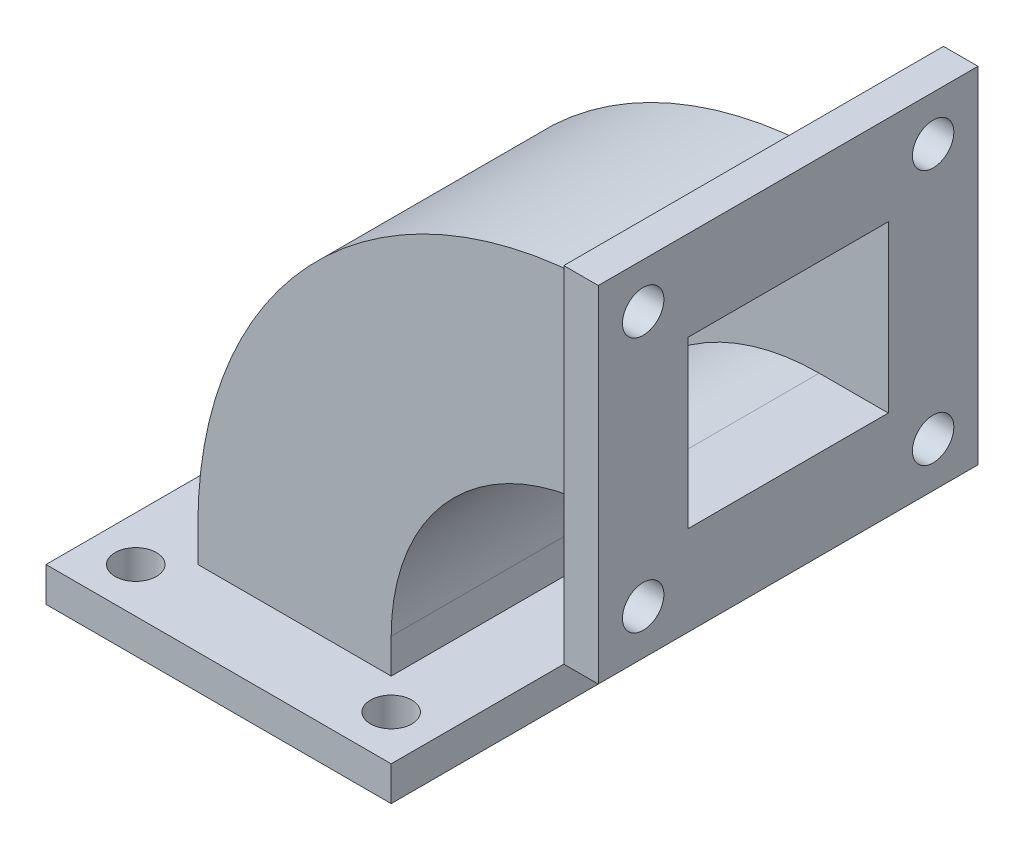
ISO-10303-21;
HEADER;
FILE_DESCRIPTION(('STEP AP214'),'2;1');
FILE_NAME('part.step','',(''),(''),'','','');
FILE_SCHEMA(('AUTOMOTIVE_DESIGN { 1 0 10303 214 1 1 1 1 }'));
ENDSEC;
DATA;
#1=APPLICATION_CONTEXT('core data for automotive mechanical design processes');
#2=APPLICATION_PROTOCOL_DEFINITION('international standard','automotive_design',2000,#1);
#3=PRODUCT_CONTEXT('',#1,'mechanical');
#4=PRODUCT('Part','Part','',(#3));
#5=PRODUCT_RELATED_PRODUCT_CATEGORY('part','',(#4));
#6=PRODUCT_DEFINITION_FORMATION('','',#4);
#7=PRODUCT_DEFINITION_CONTEXT('part definition',#1,'design');
#8=PRODUCT_DEFINITION('design','',#6,#7);
#9=PRODUCT_DEFINITION_SHAPE('','',#8);
#10=(LENGTH_UNIT() NAMED_UNIT(*) SI_UNIT(.MILLI.,.METRE.));
#11=(NAMED_UNIT(*) PLANE_ANGLE_UNIT() SI_UNIT($,.RADIAN.));
#12=(NAMED_UNIT(*) SI_UNIT($,.STERADIAN.) SOLID_ANGLE_UNIT());
#13=UNCERTAINTY_MEASURE_WITH_UNIT(LENGTH_MEASURE(1.E-05),#10,'distance_accuracy_value','');
#14=(GEOMETRIC_REPRESENTATION_CONTEXT(3) GLOBAL_UNCERTAINTY_ASSIGNED_CONTEXT((#13)) GLOBAL_UNIT_ASSIGNED_CONTEXT((#10,
#11,#12)) REPRESENTATION_CONTEXT('',''));
#15=CARTESIAN_POINT('',(0.,0.,0.));
#16=DIRECTION('',(0.,0.,1.));
#17=DIRECTION('',(1.,0.,0.));
#18=AXIS2_PLACEMENT_3D('',#15,#16,#17);
#19=CARTESIAN_POINT('',(5.,0.,0.));
#20=DIRECTION('',(1.,0.,0.));
#21=DIRECTION('',(0.,0.,-1.));
#22=AXIS2_PLACEMENT_3D('',#19,#20,#21);
#23=PLANE('',#22);
#24=CARTESIAN_POINT('',(5.,-18.5,-21.));
#25=DIRECTION('',(1.,0.,0.));
#26=DIRECTION('',(0.,0.,-1.));
#27=AXIS2_PLACEMENT_3D('',#24,#25,#26);
#28=CIRCLE('',#27,2.99999999999999);
#29=CARTESIAN_POINT('',(5.,-18.5,-24.));
#30=VERTEX_POINT('',#29);
#31=EDGE_CURVE('E380',#30,#30,#28,.T.);
#32=ORIENTED_EDGE('',*,*,#31,.F.);
#33=EDGE_LOOP('',(#32));
#34=FACE_BOUND('',#33,.T.);
#35=CARTESIAN_POINT('',(5.,18.5,21.));
#36=DIRECTION('',(1.,0.,0.));
#37=DIRECTION('',(0.,0.,-1.));
#38=AXIS2_PLACEMENT_3D('',#35,#36,#37);
#39=CIRCLE('',#38,3.);
#40=CARTESIAN_POINT('',(5.,18.5,18.));
#41=VERTEX_POINT('',#40);
#42=EDGE_CURVE('E386',#41,#41,#39,.T.);
#43=ORIENTED_EDGE('',*,*,#42,.F.);
#44=EDGE_LOOP('',(#43));
#45=FACE_BOUND('',#44,.T.);
#46=DIRECTION('',(0.,1.,0.));
#47=VECTOR('',#46,1.);
#48=CARTESIAN_POINT('',(5.,25.,-27.5));
#49=LINE('',#48,#47);
#50=CARTESIAN_POINT('',(5.,-25.,-27.5));
#51=VERTEX_POINT('',#50);
#52=CARTESIAN_POINT('',(5.,25.,-27.5));
#53=VERTEX_POINT('',#52);
#54=EDGE_CURVE('E410',#51,#53,#49,.T.);
#55=ORIENTED_EDGE('',*,*,#54,.T.);
#56=DIRECTION('',(0.,0.,1.));
#57=VECTOR('',#56,1.);
#58=CARTESIAN_POINT('',(5.,25.,27.5));
#59=LINE('',#58,#57);
#60=CARTESIAN_POINT('',(5.,25.,27.5));
#61=VERTEX_POINT('',#60);
#62=EDGE_CURVE('E414',#53,#61,#59,.T.);
#63=ORIENTED_EDGE('',*,*,#62,.T.);
#64=DIRECTION('',(0.,-1.,0.));
#65=VECTOR('',#64,1.);
#66=CARTESIAN_POINT('',(5.,25.,27.5));
#67=LINE('',#66,#65);
#68=CARTESIAN_POINT('',(5.,-25.,27.5));
#69=VERTEX_POINT('',#68);
#70=EDGE_CURVE('E418',#61,#69,#67,.T.);
#71=ORIENTED_EDGE('',*,*,#70,.T.);
#72=DIRECTION('',(0.,0.,-1.));
#73=VECTOR('',#72,1.);
#74=CARTESIAN_POINT('',(5.,-25.,27.5));
#75=LINE('',#74,#73);
#76=EDGE_CURVE('E416',#69,#51,#75,.T.);
#77=ORIENTED_EDGE('',*,*,#76,.T.);
#78=EDGE_LOOP('',(#55,#63,#71,#77));
#79=FACE_BOUND('',#78,.T.);
#80=DIRECTION('',(0.,0.,1.));
#81=VECTOR('',#80,1.);
#82=CARTESIAN_POINT('',(5.,12.,14.5));
#83=LINE('',#82,#81);
#84=CARTESIAN_POINT('',(5.,12.,-14.5));
#85=VERTEX_POINT('',#84);
#86=CARTESIAN_POINT('',(5.,12.,14.5));
#87=VERTEX_POINT('',#86);
#88=EDGE_CURVE('E396',#85,#87,#83,.T.);
#89=ORIENTED_EDGE('',*,*,#88,.F.);
#90=DIRECTION('',(0.,1.,0.));
#91=VECTOR('',#90,1.);
#92=CARTESIAN_POINT('',(5.,12.,-14.5));
#93=LINE('',#92,#91);
#94=CARTESIAN_POINT('',(5.,-12.,-14.5));
#95=VERTEX_POINT('',#94);
#96=EDGE_CURVE('E392',#95,#85,#93,.T.);
#97=ORIENTED_EDGE('',*,*,#96,.F.);
#98=DIRECTION('',(0.,0.,-1.));
#99=VECTOR('',#98,1.);
#100=CARTESIAN_POINT('',(5.,-12.,14.5));
#101=LINE('',#100,#99);
#102=CARTESIAN_POINT('',(5.,-12.,14.5));
#103=VERTEX_POINT('',#102);
#104=EDGE_CURVE('E400',#103,#95,#101,.T.);
#105=ORIENTED_EDGE('',*,*,#104,.F.);
#106=DIRECTION('',(0.,-1.,0.));
#107=VECTOR('',#106,1.);
#108=CARTESIAN_POINT('',(5.,12.,14.5));
#109=LINE('',#108,#107);
#110=EDGE_CURVE('E399',#87,#103,#109,.T.);
#111=ORIENTED_EDGE('',*,*,#110,.F.);
#112=EDGE_LOOP('',(#89,#97,#105,#111));
#113=FACE_BOUND('',#112,.T.);
#114=CARTESIAN_POINT('',(5.,18.5,-21.));
#115=DIRECTION('',(1.,0.,0.));
#116=DIRECTION('',(0.,0.,-1.));
#117=AXIS2_PLACEMENT_3D('',#114,#115,#116);
#118=CIRCLE('',#117,3.);
#119=CARTESIAN_POINT('',(5.,18.5,-24.));
#120=VERTEX_POINT('',#119);
#121=EDGE_CURVE('E382',#120,#120,#118,.T.);
#122=ORIENTED_EDGE('',*,*,#121,.F.);
#123=EDGE_LOOP('',(#122));
#124=FACE_BOUND('',#123,.T.);
#125=CARTESIAN_POINT('',(5.,-18.5,21.));
#126=DIRECTION('',(1.,0.,0.));
#127=DIRECTION('',(0.,0.,-1.));
#128=AXIS2_PLACEMENT_3D('',#125,#126,#127);
#129=CIRCLE('',#128,3.);
#130=CARTESIAN_POINT('',(5.,-18.5,18.));
#131=VERTEX_POINT('',#130);
#132=EDGE_CURVE('E371',#131,#131,#129,.T.);
#133=ORIENTED_EDGE('',*,*,#132,.F.);
#134=EDGE_LOOP('',(#133));
#135=FACE_BOUND('',#134,.T.);
#136=ADVANCED_FACE('F44',(#34,#45,#79,#113,#124,#135),#23,.T.);
#137=CARTESIAN_POINT('',(0.,0.,0.));
#138=DIRECTION('',(1.,0.,0.));
#139=DIRECTION('',(0.,0.,-1.));
#140=AXIS2_PLACEMENT_3D('',#137,#138,#139);
#141=PLANE('',#140);
#142=DIRECTION('',(0.,1.,0.));
#143=VECTOR('',#142,1.);
#144=CARTESIAN_POINT('',(0.,-50.,-16.5));
#145=LINE('',#144,#143);
#146=CARTESIAN_POINT('',(0.,-14.,-16.5));
#147=VERTEX_POINT('',#146);
#148=CARTESIAN_POINT('',(0.,14.,-16.5));
#149=VERTEX_POINT('',#148);
#150=EDGE_CURVE('E351',#147,#149,#145,.T.);
#151=ORIENTED_EDGE('',*,*,#150,.T.);
#152=DIRECTION('',(0.,0.,1.));
#153=VECTOR('',#152,1.);
#154=CARTESIAN_POINT('',(0.,14.,0.));
#155=LINE('',#154,#153);
#156=CARTESIAN_POINT('',(0.,14.,16.5));
#157=VERTEX_POINT('',#156);
#158=EDGE_CURVE('E344',#149,#157,#155,.T.);
#159=ORIENTED_EDGE('',*,*,#158,.T.);
#160=DIRECTION('',(0.,-1.,0.));
#161=VECTOR('',#160,1.);
#162=CARTESIAN_POINT('',(0.,-50.,16.5));
#163=LINE('',#162,#161);
#164=CARTESIAN_POINT('',(0.,-14.,16.5));
#165=VERTEX_POINT('',#164);
#166=EDGE_CURVE('E342',#157,#165,#163,.T.);
#167=ORIENTED_EDGE('',*,*,#166,.T.);
#168=DIRECTION('',(0.,0.,-1.));
#169=VECTOR('',#168,1.);
#170=CARTESIAN_POINT('',(0.,-14.,0.));
#171=LINE('',#170,#169);
#172=EDGE_CURVE('E349',#165,#147,#171,.T.);
#173=ORIENTED_EDGE('',*,*,#172,.T.);
#174=EDGE_LOOP('',(#151,#159,#167,#173));
#175=FACE_BOUND('',#174,.T.);
#176=DIRECTION('',(0.,1.,0.));
#177=VECTOR('',#176,1.);
#178=CARTESIAN_POINT('',(0.,25.,-27.5));
#179=LINE('',#178,#177);
#180=CARTESIAN_POINT('',(0.,-25.,-27.5));
#181=VERTEX_POINT('',#180);
#182=CARTESIAN_POINT('',(0.,25.,-27.5));
#183=VERTEX_POINT('',#182);
#184=EDGE_CURVE('E408',#181,#183,#179,.T.);
#185=ORIENTED_EDGE('',*,*,#184,.F.);
#186=DIRECTION('',(0.,0.,-1.));
#187=VECTOR('',#186,1.);
#188=CARTESIAN_POINT('',(0.,-25.,27.5));
#189=LINE('',#188,#187);
#190=CARTESIAN_POINT('',(0.,-25.,27.5));
#191=VERTEX_POINT('',#190);
#192=EDGE_CURVE('E413',#191,#181,#189,.T.);
#193=ORIENTED_EDGE('',*,*,#192,.F.);
#194=DIRECTION('',(0.,-1.,0.));
#195=VECTOR('',#194,1.);
#196=CARTESIAN_POINT('',(0.,25.,27.5));
#197=LINE('',#196,#195);
#198=CARTESIAN_POINT('',(0.,25.,27.5));
#199=VERTEX_POINT('',#198);
#200=EDGE_CURVE('E422',#199,#191,#197,.T.);
#201=ORIENTED_EDGE('',*,*,#200,.F.);
#202=DIRECTION('',(0.,0.,1.));
#203=VECTOR('',#202,1.);
#204=CARTESIAN_POINT('',(0.,25.,27.5));
#205=LINE('',#204,#203);
#206=EDGE_CURVE('E421',#183,#199,#205,.T.);
#207=ORIENTED_EDGE('',*,*,#206,.F.);
#208=EDGE_LOOP('',(#185,#193,#201,#207));
#209=FACE_BOUND('',#208,.T.);
#210=CARTESIAN_POINT('',(0.,18.5,21.));
#211=DIRECTION('',(1.,0.,0.));
#212=DIRECTION('',(0.,0.,-1.));
#213=AXIS2_PLACEMENT_3D('',#210,#211,#212);
#214=CIRCLE('',#213,3.);
#215=CARTESIAN_POINT('',(0.,18.5,18.));
#216=VERTEX_POINT('',#215);
#217=EDGE_CURVE('E387',#216,#216,#214,.T.);
#218=ORIENTED_EDGE('',*,*,#217,.T.);
#219=EDGE_LOOP('',(#218));
#220=FACE_BOUND('',#219,.T.);
#221=CARTESIAN_POINT('',(0.,18.5,-21.));
#222=DIRECTION('',(1.,0.,0.));
#223=DIRECTION('',(0.,0.,-1.));
#224=AXIS2_PLACEMENT_3D('',#221,#222,#223);
#225=CIRCLE('',#224,3.);
#226=CARTESIAN_POINT('',(0.,18.5,-24.));
#227=VERTEX_POINT('',#226);
#228=EDGE_CURVE('E379',#227,#227,#225,.T.);
#229=ORIENTED_EDGE('',*,*,#228,.T.);
#230=EDGE_LOOP('',(#229));
#231=FACE_BOUND('',#230,.T.);
#232=CARTESIAN_POINT('',(0.,-18.5,-21.));
#233=DIRECTION('',(1.,0.,0.));
#234=DIRECTION('',(0.,0.,-1.));
#235=AXIS2_PLACEMENT_3D('',#232,#233,#234);
#236=CIRCLE('',#235,2.99999999999999);
#237=CARTESIAN_POINT('',(0.,-18.5,-24.));
#238=VERTEX_POINT('',#237);
#239=EDGE_CURVE('E372',#238,#238,#236,.T.);
#240=ORIENTED_EDGE('',*,*,#239,.T.);
#241=EDGE_LOOP('',(#240));
#242=FACE_BOUND('',#241,.T.);
#243=CARTESIAN_POINT('',(0.,-18.5,21.));
#244=DIRECTION('',(1.,0.,0.));
#245=DIRECTION('',(0.,0.,-1.));
#246=AXIS2_PLACEMENT_3D('',#243,#244,#245);
#247=CIRCLE('',#246,3.);
#248=CARTESIAN_POINT('',(0.,-18.5,18.));
#249=VERTEX_POINT('',#248);
#250=EDGE_CURVE('E367',#249,#249,#247,.T.);
#251=ORIENTED_EDGE('',*,*,#250,.T.);
#252=EDGE_LOOP('',(#251));
#253=FACE_BOUND('',#252,.T.);
#254=ADVANCED_FACE('F444',(#175,#209,#220,#231,#242,#253),#141,.F.);
#255=CARTESIAN_POINT('',(5.,25.,-27.5));
#256=DIRECTION('',(0.,0.,1.));
#257=DIRECTION('',(0.,-1.,0.));
#258=AXIS2_PLACEMENT_3D('',#255,#256,#257);
#259=PLANE('',#258);
#260=ORIENTED_EDGE('',*,*,#184,.T.);
#261=DIRECTION('',(-1.,0.,0.));
#262=VECTOR('',#261,1.);
#263=CARTESIAN_POINT('',(5.,25.,-27.5));
#264=LINE('',#263,#262);
#265=EDGE_CURVE('E11',#53,#183,#264,.T.);
#266=ORIENTED_EDGE('',*,*,#265,.F.);
#267=ORIENTED_EDGE('',*,*,#54,.F.);
#268=DIRECTION('',(-1.,0.,0.));
#269=VECTOR('',#268,1.);
#270=CARTESIAN_POINT('',(5.,-25.,-27.5));
#271=LINE('',#270,#269);
#272=EDGE_CURVE('E419',#51,#181,#271,.T.);
#273=ORIENTED_EDGE('',*,*,#272,.T.);
#274=EDGE_LOOP('',(#260,#266,#267,#273));
#275=FACE_BOUND('',#274,.T.);
#276=ADVANCED_FACE('F50',(#275),#259,.F.);
#277=CARTESIAN_POINT('',(5.,25.,27.5));
#278=DIRECTION('',(0.,-1.,0.));
#279=DIRECTION('',(0.,0.,-1.));
#280=AXIS2_PLACEMENT_3D('',#277,#278,#279);
#281=PLANE('',#280);
#282=ORIENTED_EDGE('',*,*,#206,.T.);
#283=DIRECTION('',(-1.,0.,0.));
#284=VECTOR('',#283,1.);
#285=CARTESIAN_POINT('',(5.,25.,27.5));
#286=LINE('',#285,#284);
#287=EDGE_CURVE('E52',#61,#199,#286,.T.);
#288=ORIENTED_EDGE('',*,*,#287,.F.);
#289=ORIENTED_EDGE('',*,*,#62,.F.);
#290=ORIENTED_EDGE('',*,*,#265,.T.);
#291=EDGE_LOOP('',(#282,#288,#289,#290));
#292=FACE_BOUND('',#291,.T.);
#293=ADVANCED_FACE('F453',(#292),#281,.F.);
#294=CARTESIAN_POINT('',(5.,25.,27.5));
#295=DIRECTION('',(0.,0.,-1.));
#296=DIRECTION('',(0.,1.,0.));
#297=AXIS2_PLACEMENT_3D('',#294,#295,#296);
#298=PLANE('',#297);
#299=ORIENTED_EDGE('',*,*,#200,.T.);
#300=DIRECTION('',(-1.,0.,0.));
#301=VECTOR('',#300,1.);
#302=CARTESIAN_POINT('',(5.,-25.,27.5));
#303=LINE('',#302,#301);
#304=EDGE_CURVE('E429',#69,#191,#303,.T.);
#305=ORIENTED_EDGE('',*,*,#304,.F.);
#306=ORIENTED_EDGE('',*,*,#70,.F.);
#307=ORIENTED_EDGE('',*,*,#287,.T.);
#308=EDGE_LOOP('',(#299,#305,#306,#307));
#309=FACE_BOUND('',#308,.T.);
#310=ADVANCED_FACE('F440',(#309),#298,.F.);
#311=CARTESIAN_POINT('',(5.,-25.,27.5));
#312=DIRECTION('',(0.,1.,0.));
#313=DIRECTION('',(0.,0.,1.));
#314=AXIS2_PLACEMENT_3D('',#311,#312,#313);
#315=PLANE('',#314);
#316=ORIENTED_EDGE('',*,*,#192,.T.);
#317=ORIENTED_EDGE('',*,*,#272,.F.);
#318=ORIENTED_EDGE('',*,*,#76,.F.);
#319=ORIENTED_EDGE('',*,*,#304,.T.);
#320=EDGE_LOOP('',(#316,#317,#318,#319));
#321=FACE_BOUND('',#320,.T.);
#322=ADVANCED_FACE('F447',(#321),#315,.F.);
#323=CARTESIAN_POINT('',(5.,12.,-14.5));
#324=DIRECTION('',(0.,0.,1.));
#325=DIRECTION('',(0.,-1.,0.));
#326=AXIS2_PLACEMENT_3D('',#323,#324,#325);
#327=PLANE('',#326);
#328=DIRECTION('',(-1.,0.,0.));
#329=VECTOR('',#328,1.);
#330=CARTESIAN_POINT('',(5.,12.,-14.5));
#331=LINE('',#330,#329);
#332=CARTESIAN_POINT('',(-4.99999999999959,12.0000000000004,-14.5));
#333=VERTEX_POINT('',#332);
#334=EDGE_CURVE('E407',#85,#333,#331,.T.);
#335=ORIENTED_EDGE('',*,*,#334,.T.);
#336=CARTESIAN_POINT('',(-4.99999999999999,-45.,-14.5));
#337=DIRECTION('',(0.,0.,-1.));
#338=DIRECTION('',(-1.,0.,0.));
#339=AXIS2_PLACEMENT_3D('',#336,#337,#338);
#340=CIRCLE('',#339,57.0000000000003);
#341=CARTESIAN_POINT('',(-62.,-45.0000000000003,-14.5));
#342=VERTEX_POINT('',#341);
#343=EDGE_CURVE('E217',#342,#333,#340,.T.);
#344=ORIENTED_EDGE('',*,*,#343,.F.);
#345=DIRECTION('',(0.,1.,0.));
#346=VECTOR('',#345,1.);
#347=CARTESIAN_POINT('',(-62.,-50.,-14.5));
#348=LINE('',#347,#346);
#349=CARTESIAN_POINT('',(-62.,-55.,-14.5));
#350=VERTEX_POINT('',#349);
#351=EDGE_CURVE('E221',#350,#342,#348,.T.);
#352=ORIENTED_EDGE('',*,*,#351,.F.);
#353=DIRECTION('',(-1.,0.,0.));
#354=VECTOR('',#353,1.);
#355=CARTESIAN_POINT('',(-62.,-55.,-14.5));
#356=LINE('',#355,#354);
#357=CARTESIAN_POINT('',(-38.,-55.,-14.5));
#358=VERTEX_POINT('',#357);
#359=EDGE_CURVE('E222',#358,#350,#356,.T.);
#360=ORIENTED_EDGE('',*,*,#359,.F.);
#361=DIRECTION('',(0.,1.,0.));
#362=VECTOR('',#361,1.);
#363=CARTESIAN_POINT('',(-38.,-50.,-14.5));
#364=LINE('',#363,#362);
#365=CARTESIAN_POINT('',(-38.,-45.0000000000003,-14.5));
#366=VERTEX_POINT('',#365);
#367=EDGE_CURVE('E210',#358,#366,#364,.T.);
#368=ORIENTED_EDGE('',*,*,#367,.T.);
#369=CARTESIAN_POINT('',(-4.99999999999999,-45.,-14.5));
#370=DIRECTION('',(0.,0.,-1.));
#371=DIRECTION('',(-1.,0.,0.));
#372=AXIS2_PLACEMENT_3D('',#369,#370,#371);
#373=CIRCLE('',#372,33.0000000000003);
#374=CARTESIAN_POINT('',(-4.99999999999975,-11.9999999999997,-14.5));
#375=VERTEX_POINT('',#374);
#376=EDGE_CURVE('E298',#366,#375,#373,.T.);
#377=ORIENTED_EDGE('',*,*,#376,.T.);
#378=DIRECTION('',(-1.,0.,0.));
#379=VECTOR('',#378,1.);
#380=CARTESIAN_POINT('',(5.,-12.,-14.5));
#381=LINE('',#380,#379);
#382=EDGE_CURVE('E405',#95,#375,#381,.T.);
#383=ORIENTED_EDGE('',*,*,#382,.F.);
#384=ORIENTED_EDGE('',*,*,#96,.T.);
#385=EDGE_LOOP('',(#335,#344,#352,#360,#368,#377,#383,#384));
#386=FACE_BOUND('',#385,.T.);
#387=ADVANCED_FACE('F225',(#386),#327,.T.);
#388=CARTESIAN_POINT('',(5.,12.,14.5));
#389=DIRECTION('',(0.,-1.,0.));
#390=DIRECTION('',(0.,0.,-1.));
#391=AXIS2_PLACEMENT_3D('',#388,#389,#390);
#392=PLANE('',#391);
#393=DIRECTION('',(-1.,0.,0.));
#394=VECTOR('',#393,1.);
#395=CARTESIAN_POINT('',(5.,12.,14.5));
#396=LINE('',#395,#394);
#397=CARTESIAN_POINT('',(-4.99999999999959,12.0000000000004,14.5));
#398=VERTEX_POINT('',#397);
#399=EDGE_CURVE('E403',#87,#398,#396,.T.);
#400=ORIENTED_EDGE('',*,*,#399,.T.);
#401=DIRECTION('',(0.,0.,1.));
#402=VECTOR('',#401,1.);
#403=CARTESIAN_POINT('',(-4.99999999999959,12.,-14.5));
#404=LINE('',#403,#402);
#405=EDGE_CURVE('E284',#333,#398,#404,.T.);
#406=ORIENTED_EDGE('',*,*,#405,.F.);
#407=ORIENTED_EDGE('',*,*,#334,.F.);
#408=ORIENTED_EDGE('',*,*,#88,.T.);
#409=EDGE_LOOP('',(#400,#406,#407,#408));
#410=FACE_BOUND('',#409,.T.);
#411=ADVANCED_FACE('F479',(#410),#392,.T.);
#412=CARTESIAN_POINT('',(5.,12.,14.5));
#413=DIRECTION('',(0.,0.,-1.));
#414=DIRECTION('',(0.,1.,0.));
#415=AXIS2_PLACEMENT_3D('',#412,#413,#414);
#416=PLANE('',#415);
#417=DIRECTION('',(-1.,0.,0.));
#418=VECTOR('',#417,1.);
#419=CARTESIAN_POINT('',(5.,-12.,14.5));
#420=LINE('',#419,#418);
#421=CARTESIAN_POINT('',(-4.99999999999975,-11.9999999999997,14.5));
#422=VERTEX_POINT('',#421);
#423=EDGE_CURVE('E69',#103,#422,#420,.T.);
#424=ORIENTED_EDGE('',*,*,#423,.T.);
#425=CARTESIAN_POINT('',(-4.99999999999999,-45.,14.5));
#426=DIRECTION('',(0.,0.,-1.));
#427=DIRECTION('',(-1.,0.,0.));
#428=AXIS2_PLACEMENT_3D('',#425,#426,#427);
#429=CIRCLE('',#428,33.0000000000003);
#430=CARTESIAN_POINT('',(-38.,-45.0000000000003,14.5));
#431=VERTEX_POINT('',#430);
#432=EDGE_CURVE('E288',#431,#422,#429,.T.);
#433=ORIENTED_EDGE('',*,*,#432,.F.);
#434=DIRECTION('',(0.,1.,0.));
#435=VECTOR('',#434,1.);
#436=CARTESIAN_POINT('',(-38.,-50.,14.5));
#437=LINE('',#436,#435);
#438=CARTESIAN_POINT('',(-38.,-55.,14.5));
#439=VERTEX_POINT('',#438);
#440=EDGE_CURVE('E281',#439,#431,#437,.T.);
#441=ORIENTED_EDGE('',*,*,#440,.F.);
#442=DIRECTION('',(1.,0.,0.));
#443=VECTOR('',#442,1.);
#444=CARTESIAN_POINT('',(-62.,-55.,14.5));
#445=LINE('',#444,#443);
#446=CARTESIAN_POINT('',(-62.,-55.,14.5));
#447=VERTEX_POINT('',#446);
#448=EDGE_CURVE('E234',#447,#439,#445,.T.);
#449=ORIENTED_EDGE('',*,*,#448,.F.);
#450=DIRECTION('',(0.,1.,0.));
#451=VECTOR('',#450,1.);
#452=CARTESIAN_POINT('',(-62.,-50.,14.5));
#453=LINE('',#452,#451);
#454=CARTESIAN_POINT('',(-62.,-45.0000000000003,14.5));
#455=VERTEX_POINT('',#454);
#456=EDGE_CURVE('E279',#447,#455,#453,.T.);
#457=ORIENTED_EDGE('',*,*,#456,.T.);
#458=CARTESIAN_POINT('',(-4.99999999999999,-45.,14.5));
#459=DIRECTION('',(0.,0.,-1.));
#460=DIRECTION('',(-1.,0.,0.));
#461=AXIS2_PLACEMENT_3D('',#458,#459,#460);
#462=CIRCLE('',#461,57.0000000000003);
#463=EDGE_CURVE('E286',#455,#398,#462,.T.);
#464=ORIENTED_EDGE('',*,*,#463,.T.);
#465=ORIENTED_EDGE('',*,*,#399,.F.);
#466=ORIENTED_EDGE('',*,*,#110,.T.);
#467=EDGE_LOOP('',(#424,#433,#441,#449,#457,#464,#465,#466));
#468=FACE_BOUND('',#467,.T.);
#469=ADVANCED_FACE('F482',(#468),#416,.T.);
#470=CARTESIAN_POINT('',(5.,-12.,14.5));
#471=DIRECTION('',(0.,1.,0.));
#472=DIRECTION('',(0.,0.,1.));
#473=AXIS2_PLACEMENT_3D('',#470,#471,#472);
#474=PLANE('',#473);
#475=ORIENTED_EDGE('',*,*,#382,.T.);
#476=DIRECTION('',(0.,0.,-1.));
#477=VECTOR('',#476,1.);
#478=CARTESIAN_POINT('',(-4.99999999999975,-12.,-14.5));
#479=LINE('',#478,#477);
#480=EDGE_CURVE('E293',#422,#375,#479,.T.);
#481=ORIENTED_EDGE('',*,*,#480,.F.);
#482=ORIENTED_EDGE('',*,*,#423,.F.);
#483=ORIENTED_EDGE('',*,*,#104,.T.);
#484=EDGE_LOOP('',(#475,#481,#482,#483));
#485=FACE_BOUND('',#484,.T.);
#486=ADVANCED_FACE('F489',(#485),#474,.T.);
#487=CARTESIAN_POINT('',(5.,18.5,21.));
#488=DIRECTION('',(-1.,0.,0.));
#489=DIRECTION('',(0.,0.,1.));
#490=AXIS2_PLACEMENT_3D('',#487,#488,#489);
#491=CYLINDRICAL_SURFACE('',#490,3.);
#492=ORIENTED_EDGE('',*,*,#42,.T.);
#493=EDGE_LOOP('',(#492));
#494=FACE_BOUND('',#493,.T.);
#495=ORIENTED_EDGE('',*,*,#217,.F.);
#496=EDGE_LOOP('',(#495));
#497=FACE_BOUND('',#496,.T.);
#498=ADVANCED_FACE('F497',(#494,#497),#491,.F.);
#499=CARTESIAN_POINT('',(5.,18.5,-21.));
#500=DIRECTION('',(-1.,0.,0.));
#501=DIRECTION('',(0.,0.,1.));
#502=AXIS2_PLACEMENT_3D('',#499,#500,#501);
#503=CYLINDRICAL_SURFACE('',#502,3.);
#504=ORIENTED_EDGE('',*,*,#121,.T.);
#505=EDGE_LOOP('',(#504));
#506=FACE_BOUND('',#505,.T.);
#507=ORIENTED_EDGE('',*,*,#228,.F.);
#508=EDGE_LOOP('',(#507));
#509=FACE_BOUND('',#508,.T.);
#510=ADVANCED_FACE('F496',(#506,#509),#503,.F.);
#511=CARTESIAN_POINT('',(5.,-18.5,-21.));
#512=DIRECTION('',(-1.,0.,0.));
#513=DIRECTION('',(0.,0.,1.));
#514=AXIS2_PLACEMENT_3D('',#511,#512,#513);
#515=CYLINDRICAL_SURFACE('',#514,2.99999999999999);
#516=ORIENTED_EDGE('',*,*,#31,.T.);
#517=EDGE_LOOP('',(#516));
#518=FACE_BOUND('',#517,.T.);
#519=ORIENTED_EDGE('',*,*,#239,.F.);
#520=EDGE_LOOP('',(#519));
#521=FACE_BOUND('',#520,.T.);
#522=ADVANCED_FACE('F504',(#518,#521),#515,.F.);
#523=CARTESIAN_POINT('',(5.,-18.5,21.));
#524=DIRECTION('',(-1.,0.,0.));
#525=DIRECTION('',(0.,0.,1.));
#526=AXIS2_PLACEMENT_3D('',#523,#524,#525);
#527=CYLINDRICAL_SURFACE('',#526,3.);
#528=ORIENTED_EDGE('',*,*,#132,.T.);
#529=EDGE_LOOP('',(#528));
#530=FACE_BOUND('',#529,.T.);
#531=ORIENTED_EDGE('',*,*,#250,.F.);
#532=EDGE_LOOP('',(#531));
#533=FACE_BOUND('',#532,.T.);
#534=ADVANCED_FACE('F507',(#530,#533),#527,.F.);
#535=CARTESIAN_POINT('',(-64.,-50.,-14.5));
#536=DIRECTION('',(-1.,0.,0.));
#537=DIRECTION('',(0.,0.,1.));
#538=AXIS2_PLACEMENT_3D('',#535,#536,#537);
#539=PLANE('',#538);
#540=DIRECTION('',(0.,1.,0.));
#541=VECTOR('',#540,1.);
#542=CARTESIAN_POINT('',(-64.,-50.,16.5));
#543=LINE('',#542,#541);
#544=CARTESIAN_POINT('',(-64.,-50.,16.5));
#545=VERTEX_POINT('',#544);
#546=CARTESIAN_POINT('',(-64.0000000000002,-45.0000000000001,16.5));
#547=VERTEX_POINT('',#546);
#548=EDGE_CURVE('E302',#545,#547,#543,.T.);
#549=ORIENTED_EDGE('',*,*,#548,.T.);
#550=DIRECTION('',(0.,0.,-1.));
#551=VECTOR('',#550,1.);
#552=CARTESIAN_POINT('',(-64.0000000000003,-45.0000000000003,0.));
#553=LINE('',#552,#551);
#554=CARTESIAN_POINT('',(-64.0000000000002,-45.0000000000001,-16.5));
#555=VERTEX_POINT('',#554);
#556=EDGE_CURVE('E308',#555,#547,#553,.F.);
#557=ORIENTED_EDGE('',*,*,#556,.F.);
#558=DIRECTION('',(0.,1.,0.));
#559=VECTOR('',#558,1.);
#560=CARTESIAN_POINT('',(-64.,-50.,-16.5));
#561=LINE('',#560,#559);
#562=CARTESIAN_POINT('',(-64.,-50.,-16.5));
#563=VERTEX_POINT('',#562);
#564=EDGE_CURVE('E310',#563,#555,#561,.T.);
#565=ORIENTED_EDGE('',*,*,#564,.F.);
#566=DIRECTION('',(0.,0.,1.));
#567=VECTOR('',#566,1.);
#568=CARTESIAN_POINT('',(-64.,-50.,0.));
#569=LINE('',#568,#567);
#570=EDGE_CURVE('E301',#563,#545,#569,.T.);
#571=ORIENTED_EDGE('',*,*,#570,.T.);
#572=EDGE_LOOP('',(#549,#557,#565,#571));
#573=FACE_BOUND('',#572,.T.);
#574=ADVANCED_FACE('F512',(#573),#539,.T.);
#575=CARTESIAN_POINT('',(-62.,-50.,16.5));
#576=DIRECTION('',(0.,0.,1.));
#577=DIRECTION('',(1.,0.,0.));
#578=AXIS2_PLACEMENT_3D('',#575,#576,#577);
#579=PLANE('',#578);
#580=DIRECTION('',(0.,1.,0.));
#581=VECTOR('',#580,1.);
#582=CARTESIAN_POINT('',(-36.,-50.,16.5));
#583=LINE('',#582,#581);
#584=CARTESIAN_POINT('',(-36.,-50.,16.5));
#585=VERTEX_POINT('',#584);
#586=CARTESIAN_POINT('',(-36.0000000000002,-45.0000000000001,16.5));
#587=VERTEX_POINT('',#586);
#588=EDGE_CURVE('E305',#585,#587,#583,.T.);
#589=ORIENTED_EDGE('',*,*,#588,.T.);
#590=CARTESIAN_POINT('',(-4.99999999999999,-45.,16.5));
#591=DIRECTION('',(0.,0.,1.));
#592=DIRECTION('',(1.,0.,0.));
#593=AXIS2_PLACEMENT_3D('',#590,#591,#592);
#594=CIRCLE('',#593,31.0000000000003);
#595=CARTESIAN_POINT('',(-4.99999999999979,-14.,16.5));
#596=VERTEX_POINT('',#595);
#597=EDGE_CURVE('E324',#587,#596,#594,.F.);
#598=ORIENTED_EDGE('',*,*,#597,.T.);
#599=DIRECTION('',(1.,0.,0.));
#600=VECTOR('',#599,1.);
#601=CARTESIAN_POINT('',(-4.99999999999967,-14.,16.5));
#602=LINE('',#601,#600);
#603=EDGE_CURVE('E347',#596,#165,#602,.T.);
#604=ORIENTED_EDGE('',*,*,#603,.T.);
#605=ORIENTED_EDGE('',*,*,#166,.F.);
#606=DIRECTION('',(1.,0.,0.));
#607=VECTOR('',#606,1.);
#608=CARTESIAN_POINT('',(-4.99999999999967,14.,16.5));
#609=LINE('',#608,#607);
#610=CARTESIAN_POINT('',(-4.99999999999979,14.0000000000002,16.5));
#611=VERTEX_POINT('',#610);
#612=EDGE_CURVE('E338',#611,#157,#609,.T.);
#613=ORIENTED_EDGE('',*,*,#612,.F.);
#614=CARTESIAN_POINT('',(-4.99999999999999,-45.,16.5));
#615=DIRECTION('',(0.,0.,1.));
#616=DIRECTION('',(1.,0.,0.));
#617=AXIS2_PLACEMENT_3D('',#614,#615,#616);
#618=CIRCLE('',#617,59.0000000000003);
#619=EDGE_CURVE('E325',#547,#611,#618,.F.);
#620=ORIENTED_EDGE('',*,*,#619,.F.);
#621=ORIENTED_EDGE('',*,*,#548,.F.);
#622=DIRECTION('',(1.,0.,0.));
#623=VECTOR('',#622,1.);
#624=CARTESIAN_POINT('',(0.,-50.,16.5));
#625=LINE('',#624,#623);
#626=EDGE_CURVE('E353',#545,#585,#625,.T.);
#627=ORIENTED_EDGE('',*,*,#626,.T.);
#628=EDGE_LOOP('',(#589,#598,#604,#605,#613,#620,#621,#627));
#629=FACE_BOUND('',#628,.T.);
#630=ADVANCED_FACE('F536',(#629),#579,.T.);
#631=CARTESIAN_POINT('',(-36.,-50.,-14.5));
#632=DIRECTION('',(1.,0.,0.));
#633=DIRECTION('',(0.,0.,-1.));
#634=AXIS2_PLACEMENT_3D('',#631,#632,#633);
#635=PLANE('',#634);
#636=DIRECTION('',(0.,1.,0.));
#637=VECTOR('',#636,1.);
#638=CARTESIAN_POINT('',(-36.,-50.,-16.5));
#639=LINE('',#638,#637);
#640=CARTESIAN_POINT('',(-36.,-50.,-16.5));
#641=VERTEX_POINT('',#640);
#642=CARTESIAN_POINT('',(-36.0000000000002,-45.0000000000001,-16.5));
#643=VERTEX_POINT('',#642);
#644=EDGE_CURVE('E316',#641,#643,#639,.T.);
#645=ORIENTED_EDGE('',*,*,#644,.T.);
#646=DIRECTION('',(0.,0.,-1.));
#647=VECTOR('',#646,1.);
#648=CARTESIAN_POINT('',(-36.0000000000003,-45.0000000000003,0.));
#649=LINE('',#648,#647);
#650=EDGE_CURVE('E312',#587,#643,#649,.T.);
#651=ORIENTED_EDGE('',*,*,#650,.F.);
#652=ORIENTED_EDGE('',*,*,#588,.F.);
#653=DIRECTION('',(0.,0.,-1.));
#654=VECTOR('',#653,1.);
#655=CARTESIAN_POINT('',(-36.,-50.,0.));
#656=LINE('',#655,#654);
#657=EDGE_CURVE('E357',#585,#641,#656,.T.);
#658=ORIENTED_EDGE('',*,*,#657,.T.);
#659=EDGE_LOOP('',(#645,#651,#652,#658));
#660=FACE_BOUND('',#659,.T.);
#661=ADVANCED_FACE('F535',(#660),#635,.T.);
#662=CARTESIAN_POINT('',(-62.,-50.,-16.5));
#663=DIRECTION('',(0.,0.,-1.));
#664=DIRECTION('',(-1.,0.,0.));
#665=AXIS2_PLACEMENT_3D('',#662,#663,#664);
#666=PLANE('',#665);
#667=ORIENTED_EDGE('',*,*,#564,.T.);
#668=CARTESIAN_POINT('',(-4.99999999999999,-45.,-16.5));
#669=DIRECTION('',(0.,0.,-1.));
#670=DIRECTION('',(-1.,0.,0.));
#671=AXIS2_PLACEMENT_3D('',#668,#669,#670);
#672=CIRCLE('',#671,59.0000000000003);
#673=CARTESIAN_POINT('',(-4.99999999999979,14.,-16.5));
#674=VERTEX_POINT('',#673);
#675=EDGE_CURVE('E317',#555,#674,#672,.T.);
#676=ORIENTED_EDGE('',*,*,#675,.T.);
#677=DIRECTION('',(1.,0.,0.));
#678=VECTOR('',#677,1.);
#679=CARTESIAN_POINT('',(-4.99999999999967,14.,-16.5));
#680=LINE('',#679,#678);
#681=EDGE_CURVE('E337',#674,#149,#680,.T.);
#682=ORIENTED_EDGE('',*,*,#681,.T.);
#683=ORIENTED_EDGE('',*,*,#150,.F.);
#684=DIRECTION('',(1.,0.,0.));
#685=VECTOR('',#684,1.);
#686=CARTESIAN_POINT('',(-4.99999999999967,-14.,-16.5));
#687=LINE('',#686,#685);
#688=CARTESIAN_POINT('',(-4.99999999999987,-13.9999999999998,-16.5));
#689=VERTEX_POINT('',#688);
#690=EDGE_CURVE('E58',#689,#147,#687,.T.);
#691=ORIENTED_EDGE('',*,*,#690,.F.);
#692=CARTESIAN_POINT('',(-4.99999999999999,-45.,-16.5));
#693=DIRECTION('',(0.,0.,-1.));
#694=DIRECTION('',(-1.,0.,0.));
#695=AXIS2_PLACEMENT_3D('',#692,#693,#694);
#696=CIRCLE('',#695,31.0000000000003);
#697=EDGE_CURVE('E331',#643,#689,#696,.T.);
#698=ORIENTED_EDGE('',*,*,#697,.F.);
#699=ORIENTED_EDGE('',*,*,#644,.F.);
#700=DIRECTION('',(-1.,0.,0.));
#701=VECTOR('',#700,1.);
#702=CARTESIAN_POINT('',(0.,-50.,-16.5));
#703=LINE('',#702,#701);
#704=EDGE_CURVE('E315',#641,#563,#703,.T.);
#705=ORIENTED_EDGE('',*,*,#704,.T.);
#706=EDGE_LOOP('',(#667,#676,#682,#683,#691,#698,#699,#705));
#707=FACE_BOUND('',#706,.T.);
#708=ADVANCED_FACE('F526',(#707),#666,.T.);
#709=CARTESIAN_POINT('',(-4.99999999999999,-45.,0.));
#710=DIRECTION('',(0.,0.,-1.));
#711=DIRECTION('',(-1.,0.,0.));
#712=AXIS2_PLACEMENT_3D('',#709,#710,#711);
#713=CYLINDRICAL_SURFACE('',#712,59.0000000000003);
#714=ORIENTED_EDGE('',*,*,#619,.T.);
#715=DIRECTION('',(0.,0.,1.));
#716=VECTOR('',#715,1.);
#717=CARTESIAN_POINT('',(-4.99999999999959,14.,-14.5));
#718=LINE('',#717,#716);
#719=EDGE_CURVE('E326',#674,#611,#718,.T.);
#720=ORIENTED_EDGE('',*,*,#719,.F.);
#721=ORIENTED_EDGE('',*,*,#675,.F.);
#722=ORIENTED_EDGE('',*,*,#556,.T.);
#723=EDGE_LOOP('',(#714,#720,#721,#722));
#724=FACE_BOUND('',#723,.T.);
#725=ADVANCED_FACE('F523',(#724),#713,.T.);
#726=CARTESIAN_POINT('',(-4.99999999999999,-45.,0.));
#727=DIRECTION('',(0.,0.,-1.));
#728=DIRECTION('',(-1.,0.,0.));
#729=AXIS2_PLACEMENT_3D('',#726,#727,#728);
#730=CYLINDRICAL_SURFACE('',#729,31.0000000000003);
#731=ORIENTED_EDGE('',*,*,#697,.T.);
#732=DIRECTION('',(0.,0.,-1.));
#733=VECTOR('',#732,1.);
#734=CARTESIAN_POINT('',(-4.99999999999975,-14.,-14.5));
#735=LINE('',#734,#733);
#736=EDGE_CURVE('E334',#596,#689,#735,.T.);
#737=ORIENTED_EDGE('',*,*,#736,.F.);
#738=ORIENTED_EDGE('',*,*,#597,.F.);
#739=ORIENTED_EDGE('',*,*,#650,.T.);
#740=EDGE_LOOP('',(#731,#737,#738,#739));
#741=FACE_BOUND('',#740,.T.);
#742=ADVANCED_FACE('F520',(#741),#730,.F.);
#743=CARTESIAN_POINT('',(-4.99999999999967,14.,-14.5));
#744=DIRECTION('',(0.,1.,0.));
#745=DIRECTION('',(0.,0.,1.));
#746=AXIS2_PLACEMENT_3D('',#743,#744,#745);
#747=PLANE('',#746);
#748=ORIENTED_EDGE('',*,*,#612,.T.);
#749=ORIENTED_EDGE('',*,*,#158,.F.);
#750=ORIENTED_EDGE('',*,*,#681,.F.);
#751=ORIENTED_EDGE('',*,*,#719,.T.);
#752=EDGE_LOOP('',(#748,#749,#750,#751));
#753=FACE_BOUND('',#752,.T.);
#754=ADVANCED_FACE('F517',(#753),#747,.T.);
#755=CARTESIAN_POINT('',(-4.99999999999967,-14.,-14.5));
#756=DIRECTION('',(0.,-1.,0.));
#757=DIRECTION('',(0.,0.,-1.));
#758=AXIS2_PLACEMENT_3D('',#755,#756,#757);
#759=PLANE('',#758);
#760=ORIENTED_EDGE('',*,*,#690,.T.);
#761=ORIENTED_EDGE('',*,*,#172,.F.);
#762=ORIENTED_EDGE('',*,*,#603,.F.);
#763=ORIENTED_EDGE('',*,*,#736,.T.);
#764=EDGE_LOOP('',(#760,#761,#762,#763));
#765=FACE_BOUND('',#764,.T.);
#766=ADVANCED_FACE('F511',(#765),#759,.T.);
#767=CARTESIAN_POINT('',(-62.,-50.,-14.5));
#768=DIRECTION('',(-1.,0.,0.));
#769=DIRECTION('',(0.,0.,1.));
#770=AXIS2_PLACEMENT_3D('',#767,#768,#769);
#771=PLANE('',#770);
#772=ORIENTED_EDGE('',*,*,#456,.F.);
#773=DIRECTION('',(0.,0.,1.));
#774=VECTOR('',#773,1.);
#775=CARTESIAN_POINT('',(-62.,-55.,-14.5));
#776=LINE('',#775,#774);
#777=EDGE_CURVE('E229',#350,#447,#776,.T.);
#778=ORIENTED_EDGE('',*,*,#777,.F.);
#779=ORIENTED_EDGE('',*,*,#351,.T.);
#780=DIRECTION('',(0.,0.,1.));
#781=VECTOR('',#780,1.);
#782=CARTESIAN_POINT('',(-62.,-45.0000000000003,-14.5));
#783=LINE('',#782,#781);
#784=EDGE_CURVE('E274',#342,#455,#783,.T.);
#785=ORIENTED_EDGE('',*,*,#784,.T.);
#786=EDGE_LOOP('',(#772,#778,#779,#785));
#787=FACE_BOUND('',#786,.T.);
#788=ADVANCED_FACE('F516',(#787),#771,.F.);
#789=CARTESIAN_POINT('',(-38.,-50.,-14.5));
#790=DIRECTION('',(1.,0.,0.));
#791=DIRECTION('',(0.,0.,-1.));
#792=AXIS2_PLACEMENT_3D('',#789,#790,#791);
#793=PLANE('',#792);
#794=ORIENTED_EDGE('',*,*,#367,.F.);
#795=DIRECTION('',(0.,0.,-1.));
#796=VECTOR('',#795,1.);
#797=CARTESIAN_POINT('',(-38.,-55.,-14.5));
#798=LINE('',#797,#796);
#799=EDGE_CURVE('E215',#439,#358,#798,.T.);
#800=ORIENTED_EDGE('',*,*,#799,.F.);
#801=ORIENTED_EDGE('',*,*,#440,.T.);
#802=DIRECTION('',(0.,0.,-1.));
#803=VECTOR('',#802,1.);
#804=CARTESIAN_POINT('',(-38.,-45.0000000000003,-14.5));
#805=LINE('',#804,#803);
#806=EDGE_CURVE('E214',#431,#366,#805,.T.);
#807=ORIENTED_EDGE('',*,*,#806,.T.);
#808=EDGE_LOOP('',(#794,#800,#801,#807));
#809=FACE_BOUND('',#808,.T.);
#810=ADVANCED_FACE('F207',(#809),#793,.F.);
#811=CARTESIAN_POINT('',(-4.99999999999999,-45.,0.));
#812=DIRECTION('',(0.,0.,-1.));
#813=DIRECTION('',(-1.,0.,0.));
#814=AXIS2_PLACEMENT_3D('',#811,#812,#813);
#815=CYLINDRICAL_SURFACE('',#814,57.0000000000003);
#816=ORIENTED_EDGE('',*,*,#463,.F.);
#817=ORIENTED_EDGE('',*,*,#784,.F.);
#818=ORIENTED_EDGE('',*,*,#343,.T.);
#819=ORIENTED_EDGE('',*,*,#405,.T.);
#820=EDGE_LOOP('',(#816,#817,#818,#819));
#821=FACE_BOUND('',#820,.T.);
#822=ADVANCED_FACE('F547',(#821),#815,.F.);
#823=CARTESIAN_POINT('',(-4.99999999999999,-45.,0.));
#824=DIRECTION('',(0.,0.,-1.));
#825=DIRECTION('',(-1.,0.,0.));
#826=AXIS2_PLACEMENT_3D('',#823,#824,#825);
#827=CYLINDRICAL_SURFACE('',#826,33.0000000000003);
#828=ORIENTED_EDGE('',*,*,#376,.F.);
#829=ORIENTED_EDGE('',*,*,#806,.F.);
#830=ORIENTED_EDGE('',*,*,#432,.T.);
#831=ORIENTED_EDGE('',*,*,#480,.T.);
#832=EDGE_LOOP('',(#828,#829,#830,#831));
#833=FACE_BOUND('',#832,.T.);
#834=ADVANCED_FACE('F542',(#833),#827,.T.);
#835=CARTESIAN_POINT('',(0.,-50.,0.));
#836=DIRECTION('',(0.,1.,0.));
#837=DIRECTION('',(0.,0.,1.));
#838=AXIS2_PLACEMENT_3D('',#835,#836,#837);
#839=PLANE('',#838);
#840=DIRECTION('',(0.,0.,-1.));
#841=VECTOR('',#840,1.);
#842=CARTESIAN_POINT('',(-25.,-50.,-27.5));
#843=LINE('',#842,#841);
#844=CARTESIAN_POINT('',(-25.,-50.,27.5));
#845=VERTEX_POINT('',#844);
#846=CARTESIAN_POINT('',(-25.,-50.,-27.5));
#847=VERTEX_POINT('',#846);
#848=EDGE_CURVE('E244',#845,#847,#843,.T.);
#849=ORIENTED_EDGE('',*,*,#848,.T.);
#850=DIRECTION('',(-1.,0.,0.));
#851=VECTOR('',#850,1.);
#852=CARTESIAN_POINT('',(-75.,-50.,-27.5));
#853=LINE('',#852,#851);
#854=CARTESIAN_POINT('',(-75.,-50.,-27.5));
#855=VERTEX_POINT('',#854);
#856=EDGE_CURVE('E257',#847,#855,#853,.T.);
#857=ORIENTED_EDGE('',*,*,#856,.T.);
#858=DIRECTION('',(0.,0.,1.));
#859=VECTOR('',#858,1.);
#860=CARTESIAN_POINT('',(-75.,-50.,-27.5));
#861=LINE('',#860,#859);
#862=CARTESIAN_POINT('',(-75.,-50.,27.5));
#863=VERTEX_POINT('',#862);
#864=EDGE_CURVE('E263',#855,#863,#861,.T.);
#865=ORIENTED_EDGE('',*,*,#864,.T.);
#866=DIRECTION('',(1.,0.,0.));
#867=VECTOR('',#866,1.);
#868=CARTESIAN_POINT('',(-75.,-50.,27.5));
#869=LINE('',#868,#867);
#870=EDGE_CURVE('E249',#863,#845,#869,.T.);
#871=ORIENTED_EDGE('',*,*,#870,.T.);
#872=EDGE_LOOP('',(#849,#857,#865,#871));
#873=FACE_BOUND('',#872,.T.);
#874=CARTESIAN_POINT('',(-68.5,-50.,-21.));
#875=DIRECTION('',(0.,1.,0.));
#876=DIRECTION('',(0.,0.,1.));
#877=AXIS2_PLACEMENT_3D('',#874,#875,#876);
#878=CIRCLE('',#877,3.00000000000001);
#879=CARTESIAN_POINT('',(-68.5,-50.,-18.));
#880=VERTEX_POINT('',#879);
#881=EDGE_CURVE('E240',#880,#880,#878,.T.);
#882=ORIENTED_EDGE('',*,*,#881,.F.);
#883=EDGE_LOOP('',(#882));
#884=FACE_BOUND('',#883,.T.);
#885=CARTESIAN_POINT('',(-31.5,-50.,-21.));
#886=DIRECTION('',(0.,1.,0.));
#887=DIRECTION('',(0.,0.,1.));
#888=AXIS2_PLACEMENT_3D('',#885,#886,#887);
#889=CIRCLE('',#888,3.);
#890=CARTESIAN_POINT('',(-31.5,-50.,-18.));
#891=VERTEX_POINT('',#890);
#892=EDGE_CURVE('E612',#891,#891,#889,.T.);
#893=ORIENTED_EDGE('',*,*,#892,.F.);
#894=EDGE_LOOP('',(#893));
#895=FACE_BOUND('',#894,.T.);
#896=CARTESIAN_POINT('',(-31.5,-50.,21.));
#897=DIRECTION('',(0.,1.,0.));
#898=DIRECTION('',(0.,0.,1.));
#899=AXIS2_PLACEMENT_3D('',#896,#897,#898);
#900=CIRCLE('',#899,3.);
#901=CARTESIAN_POINT('',(-31.5,-50.,24.));
#902=VERTEX_POINT('',#901);
#903=EDGE_CURVE('E607',#902,#902,#900,.T.);
#904=ORIENTED_EDGE('',*,*,#903,.F.);
#905=EDGE_LOOP('',(#904));
#906=FACE_BOUND('',#905,.T.);
#907=CARTESIAN_POINT('',(-68.5,-50.,21.));
#908=DIRECTION('',(0.,1.,0.));
#909=DIRECTION('',(0.,0.,1.));
#910=AXIS2_PLACEMENT_3D('',#907,#908,#909);
#911=CIRCLE('',#910,3.00000000000001);
#912=CARTESIAN_POINT('',(-68.5,-50.,24.));
#913=VERTEX_POINT('',#912);
#914=EDGE_CURVE('E602',#913,#913,#911,.T.);
#915=ORIENTED_EDGE('',*,*,#914,.F.);
#916=EDGE_LOOP('',(#915));
#917=FACE_BOUND('',#916,.T.);
#918=ORIENTED_EDGE('',*,*,#570,.F.);
#919=ORIENTED_EDGE('',*,*,#704,.F.);
#920=ORIENTED_EDGE('',*,*,#657,.F.);
#921=ORIENTED_EDGE('',*,*,#626,.F.);
#922=EDGE_LOOP('',(#918,#919,#920,#921));
#923=FACE_BOUND('',#922,.T.);
#924=ADVANCED_FACE('F550',(#873,#884,#895,#906,#917,#923),#839,.T.);
#925=CARTESIAN_POINT('',(-25.,-55.,-27.5));
#926=DIRECTION('',(1.,0.,0.));
#927=DIRECTION('',(0.,0.,-1.));
#928=AXIS2_PLACEMENT_3D('',#925,#926,#927);
#929=PLANE('',#928);
#930=ORIENTED_EDGE('',*,*,#848,.F.);
#931=DIRECTION('',(0.,1.,0.));
#932=VECTOR('',#931,1.);
#933=CARTESIAN_POINT('',(-25.,-55.,27.5));
#934=LINE('',#933,#932);
#935=CARTESIAN_POINT('',(-25.,-55.,27.5));
#936=VERTEX_POINT('',#935);
#937=EDGE_CURVE('E268',#936,#845,#934,.T.);
#938=ORIENTED_EDGE('',*,*,#937,.F.);
#939=DIRECTION('',(0.,0.,-1.));
#940=VECTOR('',#939,1.);
#941=CARTESIAN_POINT('',(-25.,-55.,-27.5));
#942=LINE('',#941,#940);
#943=CARTESIAN_POINT('',(-25.,-55.,-27.5));
#944=VERTEX_POINT('',#943);
#945=EDGE_CURVE('E243',#936,#944,#942,.T.);
#946=ORIENTED_EDGE('',*,*,#945,.T.);
#947=DIRECTION('',(0.,1.,0.));
#948=VECTOR('',#947,1.);
#949=CARTESIAN_POINT('',(-25.,-55.,-27.5));
#950=LINE('',#949,#948);
#951=EDGE_CURVE('E260',#944,#847,#950,.T.);
#952=ORIENTED_EDGE('',*,*,#951,.T.);
#953=EDGE_LOOP('',(#930,#938,#946,#952));
#954=FACE_BOUND('',#953,.T.);
#955=ADVANCED_FACE('F559',(#954),#929,.T.);
#956=CARTESIAN_POINT('',(-75.,-55.,27.5));
#957=DIRECTION('',(0.,0.,1.));
#958=DIRECTION('',(1.,0.,0.));
#959=AXIS2_PLACEMENT_3D('',#956,#957,#958);
#960=PLANE('',#959);
#961=ORIENTED_EDGE('',*,*,#870,.F.);
#962=DIRECTION('',(0.,1.,0.));
#963=VECTOR('',#962,1.);
#964=CARTESIAN_POINT('',(-75.,-55.,27.5));
#965=LINE('',#964,#963);
#966=CARTESIAN_POINT('',(-75.,-55.,27.5));
#967=VERTEX_POINT('',#966);
#968=EDGE_CURVE('E269',#967,#863,#965,.T.);
#969=ORIENTED_EDGE('',*,*,#968,.F.);
#970=DIRECTION('',(1.,0.,0.));
#971=VECTOR('',#970,1.);
#972=CARTESIAN_POINT('',(-75.,-55.,27.5));
#973=LINE('',#972,#971);
#974=EDGE_CURVE('E255',#967,#936,#973,.T.);
#975=ORIENTED_EDGE('',*,*,#974,.T.);
#976=ORIENTED_EDGE('',*,*,#937,.T.);
#977=EDGE_LOOP('',(#961,#969,#975,#976));
#978=FACE_BOUND('',#977,.T.);
#979=ADVANCED_FACE('F561',(#978),#960,.T.);
#980=CARTESIAN_POINT('',(-75.,-55.,-27.5));
#981=DIRECTION('',(-1.,0.,0.));
#982=DIRECTION('',(0.,0.,1.));
#983=AXIS2_PLACEMENT_3D('',#980,#981,#982);
#984=PLANE('',#983);
#985=ORIENTED_EDGE('',*,*,#864,.F.);
#986=DIRECTION('',(0.,1.,0.));
#987=VECTOR('',#986,1.);
#988=CARTESIAN_POINT('',(-75.,-55.,-27.5));
#989=LINE('',#988,#987);
#990=CARTESIAN_POINT('',(-75.,-55.,-27.5));
#991=VERTEX_POINT('',#990);
#992=EDGE_CURVE('E275',#991,#855,#989,.T.);
#993=ORIENTED_EDGE('',*,*,#992,.F.);
#994=DIRECTION('',(0.,0.,1.));
#995=VECTOR('',#994,1.);
#996=CARTESIAN_POINT('',(-75.,-55.,-27.5));
#997=LINE('',#996,#995);
#998=EDGE_CURVE('E253',#991,#967,#997,.T.);
#999=ORIENTED_EDGE('',*,*,#998,.T.);
#1000=ORIENTED_EDGE('',*,*,#968,.T.);
#1001=EDGE_LOOP('',(#985,#993,#999,#1000));
#1002=FACE_BOUND('',#1001,.T.);
#1003=ADVANCED_FACE('F567',(#1002),#984,.T.);
#1004=CARTESIAN_POINT('',(-75.,-55.,-27.5));
#1005=DIRECTION('',(0.,0.,-1.));
#1006=DIRECTION('',(-1.,0.,0.));
#1007=AXIS2_PLACEMENT_3D('',#1004,#1005,#1006);
#1008=PLANE('',#1007);
#1009=ORIENTED_EDGE('',*,*,#856,.F.);
#1010=ORIENTED_EDGE('',*,*,#951,.F.);
#1011=DIRECTION('',(-1.,0.,0.));
#1012=VECTOR('',#1011,1.);
#1013=CARTESIAN_POINT('',(-75.,-55.,-27.5));
#1014=LINE('',#1013,#1012);
#1015=EDGE_CURVE('E247',#944,#991,#1014,.T.);
#1016=ORIENTED_EDGE('',*,*,#1015,.T.);
#1017=ORIENTED_EDGE('',*,*,#992,.T.);
#1018=EDGE_LOOP('',(#1009,#1010,#1016,#1017));
#1019=FACE_BOUND('',#1018,.T.);
#1020=ADVANCED_FACE('F564',(#1019),#1008,.T.);
#1021=CARTESIAN_POINT('',(0.,-55.,0.));
#1022=DIRECTION('',(0.,1.,0.));
#1023=DIRECTION('',(0.,0.,1.));
#1024=AXIS2_PLACEMENT_3D('',#1021,#1022,#1023);
#1025=PLANE('',#1024);
#1026=CARTESIAN_POINT('',(-68.5,-55.,21.));
#1027=DIRECTION('',(0.,1.,0.));
#1028=DIRECTION('',(0.,0.,1.));
#1029=AXIS2_PLACEMENT_3D('',#1026,#1027,#1028);
#1030=CIRCLE('',#1029,3.00000000000001);
#1031=CARTESIAN_POINT('',(-68.5,-55.,24.));
#1032=VERTEX_POINT('',#1031);
#1033=EDGE_CURVE('E599',#1032,#1032,#1030,.T.);
#1034=ORIENTED_EDGE('',*,*,#1033,.T.);
#1035=EDGE_LOOP('',(#1034));
#1036=FACE_BOUND('',#1035,.T.);
#1037=CARTESIAN_POINT('',(-31.5,-55.,21.));
#1038=DIRECTION('',(0.,1.,0.));
#1039=DIRECTION('',(0.,0.,1.));
#1040=AXIS2_PLACEMENT_3D('',#1037,#1038,#1039);
#1041=CIRCLE('',#1040,3.);
#1042=CARTESIAN_POINT('',(-31.5,-55.,24.));
#1043=VERTEX_POINT('',#1042);
#1044=EDGE_CURVE('E606',#1043,#1043,#1041,.T.);
#1045=ORIENTED_EDGE('',*,*,#1044,.T.);
#1046=EDGE_LOOP('',(#1045));
#1047=FACE_BOUND('',#1046,.T.);
#1048=CARTESIAN_POINT('',(-31.5,-55.,-21.));
#1049=DIRECTION('',(0.,1.,0.));
#1050=DIRECTION('',(0.,0.,1.));
#1051=AXIS2_PLACEMENT_3D('',#1048,#1049,#1050);
#1052=CIRCLE('',#1051,3.);
#1053=CARTESIAN_POINT('',(-31.5,-55.,-18.));
#1054=VERTEX_POINT('',#1053);
#1055=EDGE_CURVE('E615',#1054,#1054,#1052,.T.);
#1056=ORIENTED_EDGE('',*,*,#1055,.T.);
#1057=EDGE_LOOP('',(#1056));
#1058=FACE_BOUND('',#1057,.T.);
#1059=CARTESIAN_POINT('',(-68.5,-55.,-21.));
#1060=DIRECTION('',(0.,1.,0.));
#1061=DIRECTION('',(0.,0.,1.));
#1062=AXIS2_PLACEMENT_3D('',#1059,#1060,#1061);
#1063=CIRCLE('',#1062,3.00000000000001);
#1064=CARTESIAN_POINT('',(-68.5,-55.,-18.));
#1065=VERTEX_POINT('',#1064);
#1066=EDGE_CURVE('E233',#1065,#1065,#1063,.T.);
#1067=ORIENTED_EDGE('',*,*,#1066,.T.);
#1068=EDGE_LOOP('',(#1067));
#1069=FACE_BOUND('',#1068,.T.);
#1070=ORIENTED_EDGE('',*,*,#448,.T.);
#1071=ORIENTED_EDGE('',*,*,#799,.T.);
#1072=ORIENTED_EDGE('',*,*,#359,.T.);
#1073=ORIENTED_EDGE('',*,*,#777,.T.);
#1074=EDGE_LOOP('',(#1070,#1071,#1072,#1073));
#1075=FACE_BOUND('',#1074,.T.);
#1076=ORIENTED_EDGE('',*,*,#945,.F.);
#1077=ORIENTED_EDGE('',*,*,#974,.F.);
#1078=ORIENTED_EDGE('',*,*,#998,.F.);
#1079=ORIENTED_EDGE('',*,*,#1015,.F.);
#1080=EDGE_LOOP('',(#1076,#1077,#1078,#1079));
#1081=FACE_BOUND('',#1080,.T.);
#1082=ADVANCED_FACE('F230',(#1036,#1047,#1058,#1069,#1075,#1081),#1025,.F.);
#1083=CARTESIAN_POINT('',(-68.5,-55.,-21.));
#1084=DIRECTION('',(0.,1.,0.));
#1085=DIRECTION('',(0.,0.,1.));
#1086=AXIS2_PLACEMENT_3D('',#1083,#1084,#1085);
#1087=CYLINDRICAL_SURFACE('',#1086,3.00000000000001);
#1088=ORIENTED_EDGE('',*,*,#1066,.F.);
#1089=EDGE_LOOP('',(#1088));
#1090=FACE_BOUND('',#1089,.T.);
#1091=ORIENTED_EDGE('',*,*,#881,.T.);
#1092=EDGE_LOOP('',(#1091));
#1093=FACE_BOUND('',#1092,.T.);
#1094=ADVANCED_FACE('F578',(#1090,#1093),#1087,.F.);
#1095=CARTESIAN_POINT('',(-31.5,-55.,-21.));
#1096=DIRECTION('',(0.,1.,0.));
#1097=DIRECTION('',(0.,0.,1.));
#1098=AXIS2_PLACEMENT_3D('',#1095,#1096,#1097);
#1099=CYLINDRICAL_SURFACE('',#1098,3.);
#1100=ORIENTED_EDGE('',*,*,#1055,.F.);
#1101=EDGE_LOOP('',(#1100));
#1102=FACE_BOUND('',#1101,.T.);
#1103=ORIENTED_EDGE('',*,*,#892,.T.);
#1104=EDGE_LOOP('',(#1103));
#1105=FACE_BOUND('',#1104,.T.);
#1106=ADVANCED_FACE('F581',(#1102,#1105),#1099,.F.);
#1107=CARTESIAN_POINT('',(-31.5,-55.,21.));
#1108=DIRECTION('',(0.,1.,0.));
#1109=DIRECTION('',(0.,0.,1.));
#1110=AXIS2_PLACEMENT_3D('',#1107,#1108,#1109);
#1111=CYLINDRICAL_SURFACE('',#1110,3.);
#1112=ORIENTED_EDGE('',*,*,#1044,.F.);
#1113=EDGE_LOOP('',(#1112));
#1114=FACE_BOUND('',#1113,.T.);
#1115=ORIENTED_EDGE('',*,*,#903,.T.);
#1116=EDGE_LOOP('',(#1115));
#1117=FACE_BOUND('',#1116,.T.);
#1118=ADVANCED_FACE('F590',(#1114,#1117),#1111,.F.);
#1119=CARTESIAN_POINT('',(-68.5,-55.,21.));
#1120=DIRECTION('',(0.,1.,0.));
#1121=DIRECTION('',(0.,0.,1.));
#1122=AXIS2_PLACEMENT_3D('',#1119,#1120,#1121);
#1123=CYLINDRICAL_SURFACE('',#1122,3.00000000000001);
#1124=ORIENTED_EDGE('',*,*,#1033,.F.);
#1125=EDGE_LOOP('',(#1124));
#1126=FACE_BOUND('',#1125,.T.);
#1127=ORIENTED_EDGE('',*,*,#914,.T.);
#1128=EDGE_LOOP('',(#1127));
#1129=FACE_BOUND('',#1128,.T.);
#1130=ADVANCED_FACE('F591',(#1126,#1129),#1123,.F.);
#1131=CLOSED_SHELL('',(#136,#254,#276,#293,#310,#322,#387,#411,#469,#486,#498,#510,#522,#534,
#574,#630,#661,#708,#725,#742,#754,#766,#788,#810,#822,#834,#924,#955,#979,#1003,#1020,#1082,
#1094,#1106,#1118,#1130));
#1132=MANIFOLD_SOLID_BREP('B2',#1131);
#1133=ADVANCED_BREP_SHAPE_REPRESENTATION('',(#18,#1132),#14);
#1134=SHAPE_DEFINITION_REPRESENTATION(#9,#1133);
ENDSEC;
END-ISO-10303-21;
